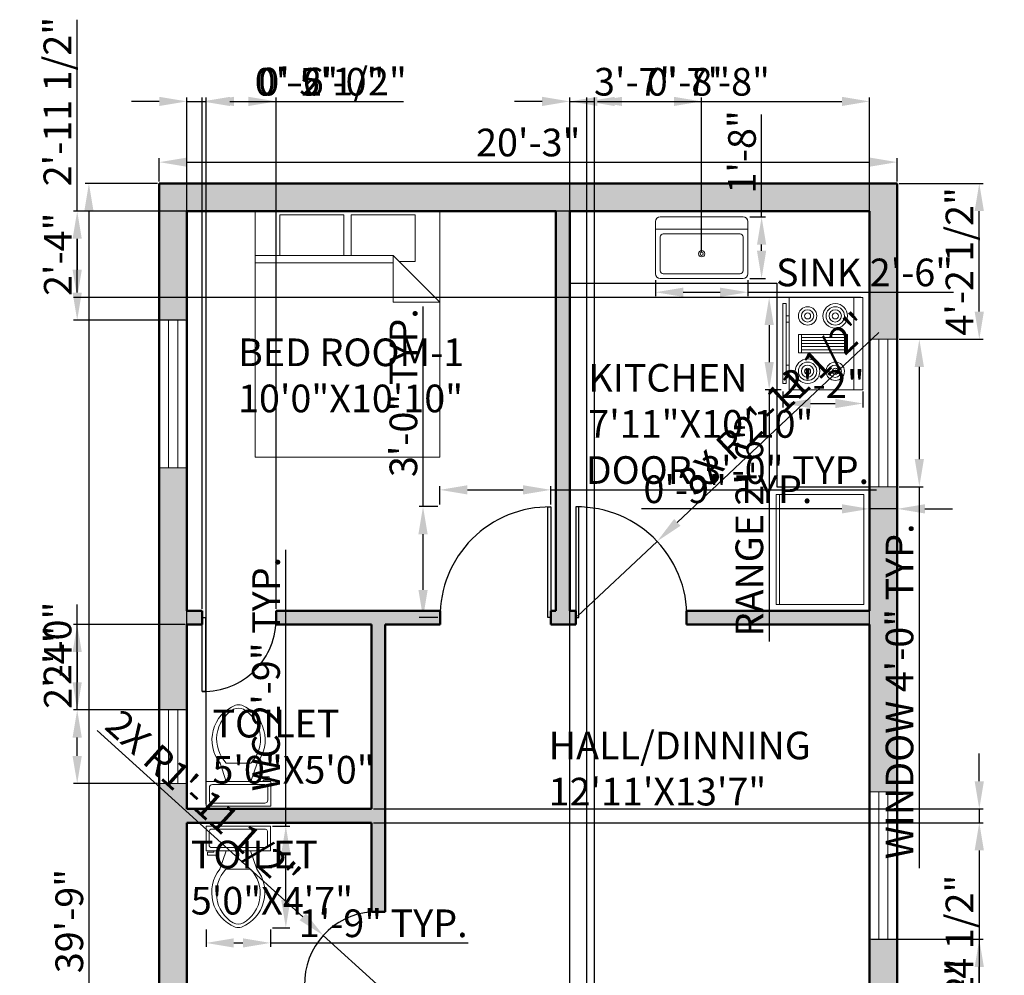
# Model space of a CAD drawing. Units: inches. Extents: x 66818 to 67138, y 29633 to 30215.
# Tile 2 of 2: x 66818 to 67138, y 29904 to 30215. Entities that reach past the tile are written whole.
import ezdxf

# ---------------------------------------------------------------- set-up
doc = ezdxf.new("R2010")
doc.units = ezdxf.units.IN
for name, color, linetype, lineweight in [('A-ANNO-DIMS', 2, 'Continuous', 18), ('A-AREA-IDEN', 7, 'Continuous', 25), ('A-DOOR', 3, 'Continuous', 25), ('A-EQPM', 8, 'Continuous', 18), ('A-FLOR-CASE', 8, 'Continuous', 25), ('A-FLOR-FIXT', 9, 'Continuous', 18), ('A-FURN', 8, 'Continuous', 18), ('A-GLAZ', 4, 'Continuous', 18), ('A-WALL', 7, 'Continuous', 50)]:
    doc.layers.add(name, color=color, linetype=linetype, lineweight=lineweight)
doc.layers.add('A-WALL-PATT', color=251, linetype='Continuous', lineweight=13, true_color=0x636466)
doc.styles.get("Standard").update_dxf_attribs({"font": 'arial.ttf'})
doc.dimstyles.new('ISO-25', dxfattribs={"dimtxt": 9, "dimasz": 9, "dimexe": 1.25, "dimexo": 0.625, "dimtad": 1, "dimdec": 1, "dimrnd": 9, "dimlunit": 3, "dimtxsty": 'Standard', "dimcen": 2.5, "dimadec": 0, "dimazin": 0, "dimtfac": 1, "dimtdec": 1, "dimtmove": 0, "dimatfit": 3, "dimfxl": 1, "dimarcsym": 0})

# ---------------------------------------------------------------- blocks, each defined once
blk = doc.blocks.new('Bed - Queen')
for p, q in [((0, -80.00003), (0, 0)), ((0, 0), (59.99999, 0)), ((59.99999, 0), (59.99999, -80.00003)), ((7.99999, -1.2), (28.79998, -1.2)), ((7.99999, -14.4), (7.99999, -1.2)), ((28.79998, -1.2), (28.79998, -14.4)), ((31.19999, -1.2), (51.99999, -1.2)), ((31.19999, -14.4), (31.19999, -1.2)), ((51.99999, -1.2), (51.99999, -16.4)), ((0, -14.4), (44.8, -14.4)), ((59.99999, -29.6), (44.8, -14.4)), ((44.8, -14.4), (44.8, -29.6)), ((44.8, -16.8), (0, -16.8)), ((51.99999, -16.4), (46.79936, -16.4)), ((44.8, -29.6), (59.99999, -29.6)), ((59.99999, -80.00003), (0, -80.00003))]:
    blk.add_line(p, q)
blk = doc.blocks.new('Toilet - top')
for p, q in [((9.5, -6), (9.5, -2)), ((-10, -8.5), (-8, -8.5)), ((-10, -9.5), (-10, -8.5)), ((-7, -9.5), (-10, -9.5)), ((-8, -8.5), (-8, -8)), ((-7, -8), (-7, -9.5)), ((-4, -8), (-6, -14)), ((4, -8), (6, -14)), ((4, -14), (-4, -14))]:
    blk.add_line(p, q)
blk.add_lwpolyline([(10.5, -8), (10.5, 0), (-10.5, 0), (-10.5, -8)], close=True)
for points in [[(-9.5, -2), (-9.5, -6)], [(8.5, -1), (-8.5, -1)], [(-8.5, -7), (8.5, -7)]]:
    blk.add_lwpolyline(points)
for centre, radius, start, end in [((-8.62, -1.88), 0.884, 81.8699, 188.1301), ((8.62, -1.88), 0.884, 351.8699, 98.1301), ((-8.62, -6.12), 0.884, 171.8699, 278.1301), ((8.62, -6.12), 0.884, 261.8699, 8.1301), ((3.52, -21.58), 12.17, 141.4691, 247.9714), ((4.2, -21.82), 11.33, 136.3677, 238.9468), ((-3.52, -21.58), 12.17, 292.0284, 38.5307), ((-4.2, -21.82), 11.33, 301.053, 43.6321), ((0, -27.88), 4, 245.7318, 294.2682), ((0, -29), 4, 254.8605, 285.1395)]:
    blk.add_arc(centre, radius, start, end)
blk = doc.blocks.new('Sink-single - 30 in top')
blk.add_line((-15, -3.999996), (15, -3.999996))
for points in [[(-13.5, 0), (13.5, 0)], [(-15, -18.499996), (-15, -1.5)], [(15, -1.5), (15, -18.499996)], [(-12.5, -5.499996), (12.5, -5.499996)], [(-13.5, -17.499996), (-13.5, -6.499996)], [(13.5, -6.499996), (13.5, -17.499996)], [(12.5, -18.499996), (-12.5, -18.499996)], [(13.5, -19.999996), (-13.5, -19.999996)]]:
    blk.add_lwpolyline(points)
for radius in [1, 0.5]:
    blk.add_circle((0, -11.999996), radius)
for centre, radius, start, end in [((-13.5, -1.5), 1.5, 90, 180), ((13.5, -1.5), 1.5, 0, 90), ((-12.5, -6.499996), 1, 90, 180), ((12.5, -6.499996), 1, 0, 90), ((-13.5, -18.499996), 1.5, 180, 270), ((-12.5, -17.499996), 1, 180, 270), ((12.5, -17.499996), 1, 270, 0), ((13.5, -18.499996), 1.5, 270, 0)]:
    blk.add_arc(centre, radius, start, end)
blk = doc.blocks.new('*D9')
at = {"layer": 'A-ANNO-DIMS', "color": 0, "lineweight": -2, "transparency": 16777216}
for p, q in [((66863.23, 30162.54), (66863.23, 30170.1)), ((67103.23, 30162.54), (67103.23, 30170.1)), ((66872.23, 30168.85), (67094.23, 30168.85))]:
    blk.add_line(p, q, dxfattribs=at)
at = {"layer": 'A-ANNO-DIMS', "color": 0, "transparency": 16777216}
for points in [[(66872.23, 30170.35), (66872.23, 30167.35), (66863.23, 30168.85)], [(67094.23, 30170.35), (67094.23, 30167.35), (67103.23, 30168.85)]]:
    blk.add_solid(points, dxfattribs=at)
at = {"layer": 'Defpoints', "color": 0, "transparency": 16777216}
for p in [(67103.23, 30168.85), (66863.23, 30161.91), (67103.23, 30161.91)]:
    blk.add_point(p, dxfattribs=at)
at = {"layer": 'A-ANNO-DIMS', "color": 0, "transparency": 16777216, "insert": (66983.23, 30174.07), "char_height": 9, "attachment_point": 5}
blk.add_mtext('20\'-3"', dxfattribs=at)
blk = doc.blocks.new('*D10')
at = {"layer": 'A-ANNO-DIMS', "color": 0, "lineweight": -2, "transparency": 16777216}
for p, q in [((66862.6, 30161.91), (66839.1, 30161.91)), ((66840.35, 30152.91), (66840.35, 29690.91)), ((66862.6, 29681.91), (66839.1, 29681.91))]:
    blk.add_line(p, q, dxfattribs=at)
at = {"layer": 'A-ANNO-DIMS', "color": 0, "transparency": 16777216}
for points in [[(66838.85, 30152.91), (66841.85, 30152.91), (66840.35, 30161.91)], [(66838.85, 29690.91), (66841.85, 29690.91), (66840.35, 29681.91)]]:
    blk.add_solid(points, dxfattribs=at)
at = {"layer": 'Defpoints', "color": 0, "transparency": 16777216}
for p in [(66863.23, 30161.91), (66840.35, 29681.91), (66863.23, 29681.91)]:
    blk.add_point(p, dxfattribs=at)
at = {"layer": 'A-ANNO-DIMS', "color": 0, "transparency": 16777216, "insert": (66835.13, 29921.91), "char_height": 9, "attachment_point": 5, "rotation": 90}
blk.add_mtext('39\'-9"', dxfattribs=at)
blk = doc.blocks.new('Range-Oven - 30 in top')
for p, q in [((0, -3), (30, -3)), ((12, -6), (18, -6)), ((13, -20), (13, -6)), ((14, -6), (14, -20)), ((15, -20), (15, -6)), ((16, -6), (16, -20)), ((17, -20), (17, -6)), ((18, -20), (12, -20)), ((6, -24), (6, -25)), ((8, -25), (8, -24)), ((22, -25), (22, -24)), ((24, -24), (24, -25))]:
    blk.add_line(p, q)
for points in [[(0, -24), (0, 0), (30, 0), (30, -24)], [(12, -21), (12, -5), (18, -5), (18, -21)], [(2, -26), (2, -25), (28, -25), (28, -26)]]:
    blk.add_lwpolyline(points, close=True)
for centre, radius in [((6, -9), 4), ((6, -9), 3), ((24, -9), 3), ((6, -9), 2), ((6, -9), 1), ((24, -9), 2), ((24, -9), 1), ((6, -18), 3), ((6, -18), 2), ((24, -18), 4), ((24, -18), 3), ((24, -18), 2), ((6, -18), 1), ((24, -18), 1)]:
    blk.add_circle(centre, radius)
blk = doc.blocks.new('WIN-48IN')
for p, q in [((9, 48), (0, 48)), ((3, 48), (3, 0)), ((6, 48), (6, 0)), ((9, 0), (0, 0))]:
    blk.add_line(p, q)
blk = doc.blocks.new('DOOR-SWING-36IN')
for p, q in [((35, 0), (35, 36)), ((35, 36), (36, 36)), ((36, 36), (36, 2.25)), ((36, 0), (35, 0))]:
    blk.add_line(p, q)
blk.add_arc((35.5, 0.5), 35.5, 89.1931, 180.8069)
blk = doc.blocks.new('*D13')
at = {"layer": 'A-ANNO-DIMS', "color": 0, "lineweight": -2, "transparency": 16777216}
for p, q in [((67103.85, 30111.23), (67111.68, 30111.23)), ((67110.43, 30102.23), (67110.43, 30072.23)), ((67103.85, 30063.23), (67111.68, 30063.23)), ((67110.43, 30063.23), (67110.43, 29939.1))]:
    blk.add_line(p, q, dxfattribs=at)
at = {"layer": 'A-ANNO-DIMS', "color": 0, "transparency": 16777216}
for points in [[(67108.93, 30102.23), (67111.93, 30102.23), (67110.43, 30111.23)], [(67108.93, 30072.23), (67111.93, 30072.23), (67110.43, 30063.23)]]:
    blk.add_solid(points, dxfattribs=at)
at = {"layer": 'Defpoints', "color": 0, "transparency": 16777216}
for p in [(67103.23, 30111.23), (67103.23, 30063.23), (67110.43, 30063.23)]:
    blk.add_point(p, dxfattribs=at)
at = {"layer": 'A-ANNO-DIMS', "color": 0, "transparency": 16777216, "insert": (67105.15, 29996.66), "char_height": 9, "attachment_point": 5, "rotation": 90}
blk.add_mtext('WINDOW 4\'-0" TYP.', dxfattribs=at)
blk = doc.blocks.new('*D14')
at = {"layer": 'A-ANNO-DIMS', "color": 0, "lineweight": -2, "transparency": 16777216}
for p, q in [((67094.23, 30062.61), (67094.23, 30054.78)), ((67103.23, 30062.61), (67103.23, 30054.78)), ((67085.23, 30056.03), (67020.12, 30056.03)), ((67103.23, 30056.03), (67094.23, 30056.03)), ((67112.23, 30056.03), (67121.23, 30056.03))]:
    blk.add_line(p, q, dxfattribs=at)
at = {"layer": 'A-ANNO-DIMS', "color": 0, "transparency": 16777216}
for points in [[(67085.23, 30057.53), (67085.23, 30054.53), (67094.23, 30056.03)], [(67112.23, 30057.53), (67112.23, 30054.53), (67103.23, 30056.03)]]:
    blk.add_solid(points, dxfattribs=at)
at = {"layer": 'Defpoints', "color": 0, "transparency": 16777216}
for p in [(67094.23, 30063.23), (67103.23, 30063.23), (67094.23, 30056.03)]:
    blk.add_point(p, dxfattribs=at)
at = {"layer": 'A-ANNO-DIMS', "color": 0, "transparency": 16777216, "insert": (67048.17, 30061.25), "char_height": 9, "attachment_point": 5}
blk.add_mtext('0\'-9" TYP.', dxfattribs=at)
blk = doc.blocks.new('*D17')
at = {"layer": 'A-ANNO-DIMS', "color": 0, "lineweight": -2, "transparency": 16777216}
for p, q in [((66904.39, 29952.81), (66904.39, 30042.72)), ((66900.06, 29952.81), (66905.64, 29952.81)), ((66904.39, 29928.76), (66904.39, 29943.81)), ((66900.06, 29919.76), (66905.64, 29919.76))]:
    blk.add_line(p, q, dxfattribs=at)
at = {"layer": 'A-ANNO-DIMS', "color": 0, "transparency": 16777216}
for points in [[(66902.89, 29943.81), (66905.89, 29943.81), (66904.39, 29952.81)], [(66902.89, 29928.76), (66905.89, 29928.76), (66904.39, 29919.76)]]:
    blk.add_solid(points, dxfattribs=at)
at = {"layer": 'Defpoints', "color": 0, "transparency": 16777216}
for p in [(66899.43, 29952.81), (66904.39, 29952.81), (66899.43, 29919.76)]:
    blk.add_point(p, dxfattribs=at)
at = {"layer": 'A-ANNO-DIMS', "color": 0, "transparency": 16777216, "insert": (66899.11, 30002.26), "char_height": 9, "attachment_point": 5, "rotation": 90}
blk.add_mtext('WC 2\'-9" TYP.', dxfattribs=at)
blk = doc.blocks.new('*D18')
at = {"layer": 'A-ANNO-DIMS', "color": 0, "lineweight": -2, "transparency": 16777216}
for p, q in [((66878.43, 29919.13), (66878.43, 29913.55)), ((66899.43, 29919.13), (66899.43, 29913.55)), ((66887.43, 29914.8), (66890.43, 29914.8)), ((66899.43, 29914.8), (66963.7, 29914.8))]:
    blk.add_line(p, q, dxfattribs=at)
at = {"layer": 'A-ANNO-DIMS', "color": 0, "transparency": 16777216}
for points in [[(66887.43, 29916.3), (66887.43, 29913.3), (66878.43, 29914.8)], [(66890.43, 29916.3), (66890.43, 29913.3), (66899.43, 29914.8)]]:
    blk.add_solid(points, dxfattribs=at)
at = {"layer": 'Defpoints', "color": 0, "transparency": 16777216}
for p in [(66878.43, 29919.76), (66899.43, 29919.76), (66899.43, 29914.8)]:
    blk.add_point(p, dxfattribs=at)
at = {"layer": 'A-ANNO-DIMS', "color": 0, "transparency": 16777216, "insert": (66936.06, 29920.02), "char_height": 9, "attachment_point": 5}
blk.add_mtext('1\'-9" TYP.', dxfattribs=at)
blk = doc.blocks.new('*D19')
at = {"layer": 'A-ANNO-DIMS', "color": 0, "lineweight": -2, "transparency": 16777216}
for p, q in [((66954.44, 30057.42), (66954.44, 30063.47)), ((66963.44, 30062.22), (66981.58, 30062.22)), ((66990.58, 30057.42), (66990.58, 30063.47)), ((66990.58, 30062.22), (67096.45, 30062.22))]:
    blk.add_line(p, q, dxfattribs=at)
at = {"layer": 'A-ANNO-DIMS', "color": 0, "transparency": 16777216}
for points in [[(66963.44, 30063.72), (66963.44, 30060.72), (66954.44, 30062.22)], [(66981.58, 30063.72), (66981.58, 30060.72), (66990.58, 30062.22)]]:
    blk.add_solid(points, dxfattribs=at)
at = {"layer": 'Defpoints', "color": 0, "transparency": 16777216}
for p in [(66990.58, 30062.22), (66954.44, 30056.8), (66990.58, 30056.8)]:
    blk.add_point(p, dxfattribs=at)
at = {"layer": 'A-ANNO-DIMS', "color": 0, "transparency": 16777216, "insert": (67048.01, 30067.5), "char_height": 9, "attachment_point": 5}
blk.add_mtext('DOOR 3\'-0" TYP.', dxfattribs=at)
blk = doc.blocks.new('*D20')
at = {"layer": 'A-ANNO-DIMS', "color": 0, "lineweight": -2, "transparency": 16777216}
for p, q in [((66949.02, 30056.8), (66949.02, 30121.9)), ((66953.82, 30056.8), (66947.77, 30056.8)), ((66949.02, 30029.66), (66949.02, 30047.8)), ((66953.82, 30020.66), (66947.77, 30020.66))]:
    blk.add_line(p, q, dxfattribs=at)
at = {"layer": 'A-ANNO-DIMS', "color": 0, "transparency": 16777216}
for points in [[(66947.52, 30047.8), (66950.52, 30047.8), (66949.02, 30056.8)], [(66947.52, 30029.66), (66950.52, 30029.66), (66949.02, 30020.66)]]:
    blk.add_solid(points, dxfattribs=at)
at = {"layer": 'Defpoints', "color": 0, "transparency": 16777216}
for p in [(66949.02, 30056.8), (66954.44, 30056.8), (66954.44, 30020.66)]:
    blk.add_point(p, dxfattribs=at)
at = {"layer": 'A-ANNO-DIMS', "color": 0, "transparency": 16777216, "insert": (66943.8, 30093.85), "char_height": 9, "attachment_point": 5, "rotation": 90}
blk.add_mtext('3\'-0" TYP.', dxfattribs=at)
blk = doc.blocks.new('*D21')
at = {"layer": 'A-ANNO-DIMS', "color": 0, "lineweight": -2, "transparency": 16777216}
for p, q in [((67024.63, 30130.4), (67024.63, 30125.27)), ((67054.63, 30130.4), (67054.63, 30125.27)), ((67033.63, 30126.52), (67045.63, 30126.52)), ((67054.63, 30126.52), (67121.6, 30126.52))]:
    blk.add_line(p, q, dxfattribs=at)
at = {"layer": 'A-ANNO-DIMS', "color": 0, "transparency": 16777216}
for points in [[(67033.63, 30128.02), (67033.63, 30125.02), (67024.63, 30126.52)], [(67045.63, 30128.02), (67045.63, 30125.02), (67054.63, 30126.52)]]:
    blk.add_solid(points, dxfattribs=at)
at = {"layer": 'Defpoints', "color": 0, "transparency": 16777216}
for p in [(67024.63, 30131.02), (67054.63, 30131.02), (67054.63, 30126.52)]:
    blk.add_point(p, dxfattribs=at)
at = {"layer": 'A-ANNO-DIMS', "color": 0, "transparency": 16777216, "insert": (67092.62, 30131.8), "char_height": 9, "attachment_point": 5}
blk.add_mtext('SINK 2\'-6"', dxfattribs=at)
blk = doc.blocks.new('*D22')
at = {"layer": 'A-ANNO-DIMS', "color": 0, "lineweight": -2, "transparency": 16777216}
for p, q in [((67059.13, 30151.02), (67059.13, 30184.35)), ((67055.26, 30151.02), (67060.38, 30151.02)), ((67059.13, 30140.02), (67059.13, 30142.02)), ((67055.26, 30131.02), (67060.38, 30131.02))]:
    blk.add_line(p, q, dxfattribs=at)
at = {"layer": 'A-ANNO-DIMS', "color": 0, "transparency": 16777216}
for points in [[(67057.63, 30142.02), (67060.63, 30142.02), (67059.13, 30151.02)], [(67057.63, 30140.02), (67060.63, 30140.02), (67059.13, 30131.02)]]:
    blk.add_solid(points, dxfattribs=at)
at = {"layer": 'Defpoints', "color": 0, "transparency": 16777216}
for p in [(67054.63, 30151.02), (67059.13, 30151.02), (67054.63, 30131.02)]:
    blk.add_point(p, dxfattribs=at)
at = {"layer": 'A-ANNO-DIMS', "color": 0, "transparency": 16777216, "insert": (67053.91, 30172.19), "char_height": 9, "attachment_point": 5, "rotation": 90}
blk.add_mtext('1\'-8"', dxfattribs=at)
blk = doc.blocks.new('*D23')
at = {"layer": 'A-ANNO-DIMS', "color": 0, "lineweight": -2, "transparency": 16777216}
for p, q in [((67065.46, 30124.82), (67060.34, 30124.82)), ((67061.59, 30115.82), (67061.59, 30103.82)), ((67065.46, 30094.82), (67060.34, 30094.82)), ((67061.59, 30094.82), (67061.59, 30012.9))]:
    blk.add_line(p, q, dxfattribs=at)
at = {"layer": 'A-ANNO-DIMS', "color": 0, "transparency": 16777216}
for points in [[(67060.09, 30115.82), (67063.09, 30115.82), (67061.59, 30124.82)], [(67060.09, 30103.82), (67063.09, 30103.82), (67061.59, 30094.82)]]:
    blk.add_solid(points, dxfattribs=at)
at = {"layer": 'Defpoints', "color": 0, "transparency": 16777216}
for p in [(67066.09, 30124.82), (67061.59, 30094.82), (67066.09, 30094.82)]:
    blk.add_point(p, dxfattribs=at)
at = {"layer": 'A-ANNO-DIMS', "color": 0, "transparency": 16777216, "insert": (67056.31, 30049.36), "char_height": 9, "attachment_point": 5, "rotation": 90}
blk.add_mtext('RANGE 2\'-6"', dxfattribs=at)
blk = doc.blocks.new('*D24')
at = {"layer": 'A-ANNO-DIMS', "color": 0, "lineweight": -2, "transparency": 16777216}
for p, q in [((67066.09, 30094.19), (67066.09, 30089.07)), ((67092.09, 30094.19), (67092.09, 30089.07)), ((67075.09, 30090.32), (67083.09, 30090.32))]:
    blk.add_line(p, q, dxfattribs=at)
at = {"layer": 'A-ANNO-DIMS', "color": 0, "transparency": 16777216}
for points in [[(67075.09, 30091.82), (67075.09, 30088.82), (67066.09, 30090.32)], [(67083.09, 30091.82), (67083.09, 30088.82), (67092.09, 30090.32)]]:
    blk.add_solid(points, dxfattribs=at)
at = {"layer": 'Defpoints', "color": 0, "transparency": 16777216}
for p in [(67066.09, 30094.82), (67092.09, 30094.82), (67092.09, 30090.32)]:
    blk.add_point(p, dxfattribs=at)
at = {"layer": 'A-ANNO-DIMS', "color": 0, "transparency": 16777216, "insert": (67079.09, 30095.46), "char_height": 9, "attachment_point": 5}
blk.add_mtext('2\'-2"', dxfattribs=at)
blk = doc.blocks.new('*D27')
at = {"layer": 'A-ANNO-DIMS', "color": 0, "lineweight": -2, "transparency": 16777216}
for p, q in [((66877.23, 30023.54), (66877.23, 30189.86)), ((66901.23, 30023.54), (66901.23, 30189.86)), ((66886.23, 30188.61), (66892.23, 30188.61)), ((66901.23, 30188.61), (66935.55, 30188.61))]:
    blk.add_line(p, q, dxfattribs=at)
at = {"layer": 'A-ANNO-DIMS', "color": 0, "transparency": 16777216}
for points in [[(66886.23, 30190.11), (66886.23, 30187.11), (66877.23, 30188.61)], [(66892.23, 30190.11), (66892.23, 30187.11), (66901.23, 30188.61)]]:
    blk.add_solid(points, dxfattribs=at)
at = {"layer": 'Defpoints', "color": 0, "transparency": 16777216}
for p in [(66901.23, 30188.61), (66877.23, 30022.91), (66901.23, 30022.91)]:
    blk.add_point(p, dxfattribs=at)
at = {"layer": 'A-ANNO-DIMS', "color": 0, "transparency": 16777216, "insert": (66922.89, 30193.83), "char_height": 9, "attachment_point": 5}
blk.add_mtext('2\'-0"', dxfattribs=at)
blk = doc.blocks.new('*D28')
at = {"layer": 'A-ANNO-DIMS', "color": 0, "lineweight": -2, "transparency": 16777216}
for p, q in [((66872.23, 30023.54), (66872.23, 30189.86)), ((66877.23, 30023.54), (66877.23, 30189.86)), ((66863.23, 30188.61), (66854.23, 30188.61)), ((66872.23, 30188.61), (66877.23, 30188.61)), ((66886.23, 30188.61), (66920.4, 30188.61))]:
    blk.add_line(p, q, dxfattribs=at)
at = {"layer": 'A-ANNO-DIMS', "color": 0, "transparency": 16777216}
for points in [[(66863.23, 30190.11), (66863.23, 30187.11), (66872.23, 30188.61)], [(66886.23, 30190.11), (66886.23, 30187.11), (66877.23, 30188.61)]]:
    blk.add_solid(points, dxfattribs=at)
at = {"layer": 'Defpoints', "color": 0, "transparency": 16777216}
for p in [(66877.23, 30188.61), (66872.23, 30022.91), (66877.23, 30022.91)]:
    blk.add_point(p, dxfattribs=at)
at = {"layer": 'A-ANNO-DIMS', "color": 0, "transparency": 16777216, "insert": (66907.81, 30193.83), "char_height": 9, "attachment_point": 5}
blk.add_mtext('0\'-5"', dxfattribs=at)
blk = doc.blocks.new('*D29')
at = {"layer": 'A-ANNO-DIMS', "color": 0, "lineweight": -2, "transparency": 16777216}
for p, q in [((67129.93, 29967.41), (67129.93, 29976.41)), ((66932.85, 29958.41), (67131.18, 29958.41)), ((67129.93, 29958.41), (67129.93, 29953.91)), ((66932.85, 29953.91), (67131.18, 29953.91)), ((67129.93, 29944.91), (67129.93, 29889.77))]:
    blk.add_line(p, q, dxfattribs=at)
at = {"layer": 'A-ANNO-DIMS', "color": 0, "transparency": 16777216}
for points in [[(67128.43, 29967.41), (67131.43, 29967.41), (67129.93, 29958.41)], [(67128.43, 29944.91), (67131.43, 29944.91), (67129.93, 29953.91)]]:
    blk.add_solid(points, dxfattribs=at)
at = {"layer": 'Defpoints', "color": 0, "transparency": 16777216}
for p in [(66932.23, 29958.41), (66932.23, 29953.91), (67129.93, 29953.91)]:
    blk.add_point(p, dxfattribs=at)
at = {"layer": 'A-ANNO-DIMS', "color": 0, "transparency": 16777216, "insert": (67124.65, 29912.84), "char_height": 9, "attachment_point": 5, "rotation": 90}
blk.add_mtext('0\'-4 1/2"', dxfattribs=at)
blk = doc.blocks.new('*D30')
at = {"layer": 'A-ANNO-DIMS', "color": 0, "lineweight": -2, "transparency": 16777216}
for p, q in [((66836.53, 30152.91), (66836.53, 30215.21)), ((66871.6, 30152.91), (66835.28, 30152.91)), ((66836.53, 30126.42), (66836.53, 30143.91)), ((66871.6, 30117.42), (66835.28, 30117.42))]:
    blk.add_line(p, q, dxfattribs=at)
at = {"layer": 'A-ANNO-DIMS', "color": 0, "transparency": 16777216}
for points in [[(66835.03, 30143.91), (66838.03, 30143.91), (66836.53, 30152.91)], [(66835.03, 30126.42), (66838.03, 30126.42), (66836.53, 30117.42)]]:
    blk.add_solid(points, dxfattribs=at)
at = {"layer": 'Defpoints', "color": 0, "transparency": 16777216}
for p in [(66836.53, 30152.91), (66872.23, 30152.91), (66872.23, 30117.42)]:
    blk.add_point(p, dxfattribs=at)
at = {"layer": 'A-ANNO-DIMS', "color": 0, "transparency": 16777216, "insert": (66831.25, 30188.56), "char_height": 9, "attachment_point": 5, "rotation": 90}
blk.add_mtext('2\'-11 1/2"', dxfattribs=at)
blk = doc.blocks.new('*D31')
at = {"layer": 'A-ANNO-DIMS', "color": 0, "lineweight": -2, "transparency": 16777216}
for p, q in [((67103.85, 30161.91), (67131.18, 30161.91)), ((67129.93, 30120.23), (67129.93, 30152.91)), ((67103.85, 30111.23), (67131.18, 30111.23))]:
    blk.add_line(p, q, dxfattribs=at)
at = {"layer": 'A-ANNO-DIMS', "color": 0, "transparency": 16777216}
for points in [[(67128.43, 30152.91), (67131.43, 30152.91), (67129.93, 30161.91)], [(67128.43, 30120.23), (67131.43, 30120.23), (67129.93, 30111.23)]]:
    blk.add_solid(points, dxfattribs=at)
at = {"layer": 'Defpoints', "color": 0, "transparency": 16777216}
for p in [(67103.23, 30161.91), (67129.93, 30161.91), (67103.23, 30111.23)]:
    blk.add_point(p, dxfattribs=at)
at = {"layer": 'A-ANNO-DIMS', "color": 0, "transparency": 16777216, "insert": (67124.65, 30136.57), "char_height": 9, "attachment_point": 5, "rotation": 90}
blk.add_mtext('4\'-2 1/2"', dxfattribs=at)
blk = doc.blocks.new('*D32')
at = {"layer": 'A-ANNO-DIMS', "color": 0, "lineweight": -2, "transparency": 16777216}
for p, q in [((67094.85, 29915.99), (67131.18, 29915.99)), ((67129.93, 29864.41), (67129.93, 29906.99)), ((67094.85, 29855.41), (67131.18, 29855.41))]:
    blk.add_line(p, q, dxfattribs=at)
at = {"layer": 'A-ANNO-DIMS', "color": 0, "transparency": 16777216}
for points in [[(67128.43, 29906.99), (67131.43, 29906.99), (67129.93, 29915.99)], [(67128.43, 29864.41), (67131.43, 29864.41), (67129.93, 29855.41)]]:
    blk.add_solid(points, dxfattribs=at)
at = {"layer": 'Defpoints', "color": 0, "transparency": 16777216}
for p in [(67094.23, 29915.99), (67129.93, 29915.99), (67094.23, 29855.41)]:
    blk.add_point(p, dxfattribs=at)
at = {"layer": 'A-ANNO-DIMS', "color": 0, "transparency": 16777216, "insert": (67124.65, 29885.7), "char_height": 9, "attachment_point": 5, "rotation": 90}
blk.add_mtext('5\'-0 1/2"', dxfattribs=at)
blk = doc.blocks.new('*D33')
at = {"layer": 'A-ANNO-DIMS', "color": 0, "lineweight": -2, "transparency": 16777216}
for p, q in [((66871.6, 30018.41), (66835.28, 30018.41)), ((66836.53, 30009.41), (66836.53, 29999.63)), ((66871.6, 29990.63), (66835.28, 29990.63))]:
    blk.add_line(p, q, dxfattribs=at)
at = {"layer": 'A-ANNO-DIMS', "color": 0, "transparency": 16777216}
for points in [[(66835.03, 30009.41), (66838.03, 30009.41), (66836.53, 30018.41)], [(66835.03, 29999.63), (66838.03, 29999.63), (66836.53, 29990.63)]]:
    blk.add_solid(points, dxfattribs=at)
at = {"layer": 'Defpoints', "color": 0, "transparency": 16777216}
for p in [(66872.23, 30018.41), (66836.53, 29990.63), (66872.23, 29990.63)]:
    blk.add_point(p, dxfattribs=at)
at = {"layer": 'A-ANNO-DIMS', "color": 0, "transparency": 16777216, "insert": (66831.39, 30004.52), "char_height": 9, "attachment_point": 5, "rotation": 90}
blk.add_mtext('2\'-4"', dxfattribs=at)
blk = doc.blocks.new('*D34')
at = {"layer": 'A-ANNO-DIMS', "color": 0, "lineweight": -2, "transparency": 16777216}
for p, q in [((66836.53, 29990.63), (66836.53, 30024.96)), ((66862.6, 29990.63), (66835.28, 29990.63)), ((66836.53, 29975.63), (66836.53, 29981.63)), ((66862.6, 29966.63), (66835.28, 29966.63))]:
    blk.add_line(p, q, dxfattribs=at)
at = {"layer": 'A-ANNO-DIMS', "color": 0, "transparency": 16777216}
for points in [[(66835.03, 29981.63), (66838.03, 29981.63), (66836.53, 29990.63)], [(66835.03, 29975.63), (66838.03, 29975.63), (66836.53, 29966.63)]]:
    blk.add_solid(points, dxfattribs=at)
at = {"layer": 'Defpoints', "color": 0, "transparency": 16777216}
for p in [(66836.53, 29990.63), (66863.23, 29990.63), (66863.23, 29966.63)]:
    blk.add_point(p, dxfattribs=at)
at = {"layer": 'A-ANNO-DIMS', "color": 0, "transparency": 16777216, "insert": (66831.31, 30012.29), "char_height": 9, "attachment_point": 5, "rotation": 90}
blk.add_mtext('2\'-0"', dxfattribs=at)
blk = doc.blocks.new('*D40')
at = {"layer": 'A-ANNO-DIMS', "color": 0, "lineweight": -2, "transparency": 16777216}
for p, q in [((66996.73, 30153.54), (66996.73, 30189.86)), ((67039.63, 30139.65), (67039.63, 30189.86)), ((67005.73, 30188.61), (67030.63, 30188.61))]:
    blk.add_line(p, q, dxfattribs=at)
at = {"layer": 'A-ANNO-DIMS', "color": 0, "transparency": 16777216}
for points in [[(67005.73, 30190.11), (67005.73, 30187.11), (66996.73, 30188.61)], [(67030.63, 30190.11), (67030.63, 30187.11), (67039.63, 30188.61)]]:
    blk.add_solid(points, dxfattribs=at)
at = {"layer": 'Defpoints', "color": 0, "transparency": 16777216}
for p in [(67039.63, 30188.61), (66996.73, 30152.91), (67039.63, 30139.02)]:
    blk.add_point(p, dxfattribs=at)
at = {"layer": 'A-ANNO-DIMS', "color": 0, "transparency": 16777216, "insert": (67018.18, 30193.84), "char_height": 9, "attachment_point": 5}
blk.add_mtext('3\'-7"', dxfattribs=at)
blk = doc.blocks.new('*D41')
at = {"layer": 'A-ANNO-DIMS', "color": 0, "lineweight": -2, "transparency": 16777216}
for p, q in [((67093.6, 30152.91), (66835.28, 30152.91)), ((66836.53, 30143.91), (66836.53, 30133.82)), ((67091.46, 30124.82), (66835.28, 30124.82))]:
    blk.add_line(p, q, dxfattribs=at)
at = {"layer": 'A-ANNO-DIMS', "color": 0, "transparency": 16777216}
for points in [[(66835.03, 30143.91), (66838.03, 30143.91), (66836.53, 30152.91)], [(66835.03, 30133.82), (66838.03, 30133.82), (66836.53, 30124.82)]]:
    blk.add_solid(points, dxfattribs=at)
at = {"layer": 'Defpoints', "color": 0, "transparency": 16777216}
for p in [(67094.23, 30152.91), (66836.53, 30124.82), (67092.09, 30124.82)]:
    blk.add_point(p, dxfattribs=at)
at = {"layer": 'A-ANNO-DIMS', "color": 0, "transparency": 16777216, "insert": (66831.39, 30138.87), "char_height": 9, "attachment_point": 5, "rotation": 90}
blk.add_mtext('2\'-4"', dxfattribs=at)
blk = doc.blocks.new('*D42')
at = {"layer": 'A-ANNO-DIMS', "color": 0, "lineweight": -2, "transparency": 16777216}
for p, q in [((66872.23, 29959.04), (66872.23, 30189.86)), ((66878.52, 29959.92), (66878.52, 30189.86)), ((66863.23, 30188.61), (66854.23, 30188.61)), ((66872.23, 30188.61), (66878.52, 30188.61)), ((66887.52, 30188.61), (66942.67, 30188.61))]:
    blk.add_line(p, q, dxfattribs=at)
at = {"layer": 'A-ANNO-DIMS', "color": 0, "transparency": 16777216}
for points in [[(66863.23, 30190.11), (66863.23, 30187.11), (66872.23, 30188.61)], [(66887.52, 30190.11), (66887.52, 30187.11), (66878.52, 30188.61)]]:
    blk.add_solid(points, dxfattribs=at)
at = {"layer": 'Defpoints', "color": 0, "transparency": 16777216}
for p in [(66878.52, 30188.61), (66878.52, 29959.3), (66872.23, 29958.41)]:
    blk.add_point(p, dxfattribs=at)
at = {"layer": 'A-ANNO-DIMS', "color": 0, "transparency": 16777216, "insert": (66919.59, 30193.89), "char_height": 9, "attachment_point": 5}
blk.add_mtext('0\'-6 1/2"', dxfattribs=at)
blk = doc.blocks.new('*D43')
at = {"layer": 'A-ANNO-DIMS', "color": 0, "lineweight": -2, "transparency": 16777216}
for p, q in [((67002.34, 29682.54), (67002.34, 30189.86)), ((67094.23, 29682.54), (67094.23, 30189.86)), ((67011.34, 30188.61), (67085.23, 30188.61))]:
    blk.add_line(p, q, dxfattribs=at)
at = {"layer": 'A-ANNO-DIMS', "color": 0, "transparency": 16777216}
for points in [[(67011.34, 30190.11), (67011.34, 30187.11), (67002.34, 30188.61)], [(67085.23, 30190.11), (67085.23, 30187.11), (67094.23, 30188.61)]]:
    blk.add_solid(points, dxfattribs=at)
at = {"layer": 'Defpoints', "color": 0, "transparency": 16777216}
for p in [(67094.23, 30188.61), (67002.34, 29681.91), (67094.23, 29681.91)]:
    blk.add_point(p, dxfattribs=at)
at = {"layer": 'A-ANNO-DIMS', "color": 0, "transparency": 16777216, "insert": (67048.28, 30193.83), "char_height": 9, "attachment_point": 5}
blk.add_mtext('7\'-8"', dxfattribs=at)
blk = doc.blocks.new('*D44')
at = {"layer": 'A-ANNO-DIMS', "color": 0, "lineweight": -2, "transparency": 16777216}
for p, q in [((66996.73, 29856.04), (66996.73, 30189.86)), ((67004.76, 29856.04), (67004.76, 30189.86)), ((66987.73, 30188.61), (66978.73, 30188.61)), ((66996.73, 30188.61), (67004.76, 30188.61)), ((67013.76, 30188.61), (67047.94, 30188.61))]:
    blk.add_line(p, q, dxfattribs=at)
at = {"layer": 'A-ANNO-DIMS', "color": 0, "transparency": 16777216}
for points in [[(66987.73, 30190.11), (66987.73, 30187.11), (66996.73, 30188.61)], [(67013.76, 30190.11), (67013.76, 30187.11), (67004.76, 30188.61)]]:
    blk.add_solid(points, dxfattribs=at)
at = {"layer": 'Defpoints', "color": 0, "transparency": 16777216}
for p in [(67004.76, 30188.61), (66996.73, 29855.41), (67004.76, 29855.41)]:
    blk.add_point(p, dxfattribs=at)
at = {"layer": 'A-ANNO-DIMS', "color": 0, "transparency": 16777216, "insert": (67035.35, 30193.83), "char_height": 9, "attachment_point": 5}
blk.add_mtext('0\'-8"', dxfattribs=at)
blk = doc.blocks.new('*D45')
at = {"layer": 'A-ANNO-DIMS', "color": 0, "lineweight": -2, "transparency": 16777216}
for p, q in [((67097.31, 30113.38), (67031.71, 30051.64)), ((66999.23, 30021.07), (67025.16, 30045.47))]:
    blk.add_line(p, q, dxfattribs=at)
at = {"layer": 'A-ANNO-DIMS', "color": 0, "transparency": 16777216}
blk.add_solid([(67030.68, 30052.73), (67032.74, 30050.54), (67025.16, 30045.47)], dxfattribs=at)
at = {"layer": 'Defpoints', "color": 0, "transparency": 16777216}
for p in [(67025.16, 30045.47), (66999.23, 30021.07)]:
    blk.add_point(p, dxfattribs=at)
at = {"layer": 'A-ANNO-DIMS', "color": 0, "transparency": 16777216, "insert": (67064.17, 30089.44), "char_height": 9, "attachment_point": 5, "rotation": 43.2645}
blk.add_mtext('3X R2\'-11 1/2"', dxfattribs=at)
blk = doc.blocks.new('*D46')
at = {"layer": 'A-ANNO-DIMS', "color": 0, "lineweight": -2, "transparency": 16777216}
for p, q in [((66843.04, 29983.89), (66909.91, 29923.29)), ((66934.04, 29901.42), (66916.58, 29917.25))]:
    blk.add_line(p, q, dxfattribs=at)
at = {"layer": 'A-ANNO-DIMS', "color": 0, "transparency": 16777216}
blk.add_solid([(66910.92, 29924.4), (66908.9, 29922.18), (66916.58, 29917.25)], dxfattribs=at)
at = {"layer": 'Defpoints', "color": 0, "transparency": 16777216}
for p in [(66916.58, 29917.25), (66934.04, 29901.42)]:
    blk.add_point(p, dxfattribs=at)
at = {"layer": 'A-ANNO-DIMS', "color": 0, "transparency": 16777216, "insert": (66876.69, 29960.52), "char_height": 9, "attachment_point": 5, "rotation": 317.8154}
blk.add_mtext('2X R1\'-11 1/2"', dxfattribs=at)

msp = doc.modelspace()

# ---------------------------------------------------------------- hatches: boundary and pattern name
at = {"layer": 'A-WALL-PATT'}
h = msp.add_hatch(color=256, dxfattribs=at)
h.dxf.hatch_style = 1
h.paths.add_polyline_path([(66872.23, 30152.91), (66992.23, 30152.91), (66992.23, 30022.91), (66990.58, 30022.91), (66990.58, 30018.41), (66998.73, 30018.41), (66998.73, 30022.91), (66996.73, 30022.91), (66996.73, 30152.91), (67094.23, 30152.91), (67094.23, 30111.23), (67103.23, 30111.23), (67103.23, 30161.91), (66863.23, 30161.91), (66863.23, 30117.42), (66872.23, 30117.42)])
h.paths.add_polyline_path([(66872.23, 30069.42), (66863.23, 30069.42), (66863.23, 29990.63), (66872.23, 29990.63), (66872.23, 30018.41), (66877.23, 30018.41), (66877.23, 30022.91), (66872.23, 30022.91)])
h.paths.add_polyline_path([(66954.58, 30020.66, -0.007042), (66954.58, 30021.66), (66954.58, 30022.91), (66901.23, 30022.91), (66901.23, 30020.66, -0.010637), (66901.23, 30019.66), (66901.23, 30018.41), (66932.23, 30018.41), (66932.23, 29958.41), (66872.23, 29958.41), (66872.23, 29966.63), (66863.23, 29966.63), (66863.23, 29867.61), (66872.23, 29867.61), (66872.23, 29894.41), (66951.63, 29894.41), (66951.63, 29895.66, -0.007042), (66951.63, 29896.66), (66951.63, 29898.91), (66936.73, 29898.91), (66936.73, 29900.92), (66932.23, 29900.92), (66932.23, 29898.91), (66872.23, 29898.91), (66872.23, 29953.91), (66932.23, 29953.91), (66932.23, 29924.92), (66936.73, 29924.92), (66936.73, 30018.41), (66954.58, 30018.41)])
h.paths.add_polyline_path([(67103.23, 30063.23), (67094.23, 30063.23), (67094.23, 30022.91), (67034.78, 30022.91, -0.031636), (67034.73, 30018.41), (67094.23, 30018.41), (67094.23, 29963.99), (67103.23, 29963.99)])
h.paths.add_polyline_path([(67103.23, 29915.99), (67094.23, 29915.99), (67094.23, 29855.41), (67040.76, 29855.41), (67040.76, 29851.91, -0.007042), (67040.76, 29850.91), (67040.76, 29846.41), (67094.23, 29846.41), (67094.23, 29690.91), (67094.23, 29681.91), (67103.23, 29681.91)])
h.paths.add_polyline_path([(67001.23, 29846.41), (67004.76, 29846.41), (67004.76, 29855.41), (66996.73, 29855.41), (66996.73, 29898.91), (66987.63, 29898.91), (66987.63, 29894.41), (66992.23, 29894.41), (66992.23, 29771.41), (66996.73, 29771.41), (66996.73, 29766.91), (67001.23, 29766.91), (67001.23, 29771.41)])
h.paths.add_polyline_path([(66872.23, 29819.61), (66863.23, 29819.61), (66863.23, 29756.49), (66872.23, 29756.49), (66872.23, 29766.91), (66996.73, 29766.91), (66996.73, 29771.41), (66872.23, 29771.41)])
h.paths.add_polyline_path([(67002.34, 29690.91), (66872.23, 29690.91), (66872.23, 29708.49), (66863.23, 29708.49), (66863.23, 29681.91), (67002.34, 29681.91)])
h.paths.add_polyline_path([(66918.07, 29755.08), (66954.6, 29755.08), (66954.6, 29773.63), (66918.07, 29773.63)], flags=9)

# ---------------------------------------------------------------- linework, layer by layer
at = {"layer": 'A-DOOR'}
for p, q in [((66999.73, 30056.66), (66998.73, 30056.66)), ((66998.73, 30056.66), (66998.73, 30022.91)), ((66999.73, 30020.66), (66999.73, 30056.66)), ((66877.23, 30020.66), (66878.23, 30020.66)), ((66878.23, 30020.66), (66878.23, 29996.66)), ((66998.73, 30020.66), (66999.73, 30020.66)), ((66877.23, 29996.66), (66877.23, 30018.41)), ((66878.23, 29996.66), (66877.23, 29996.66))]:
    msp.add_line(p, q, dxfattribs=at)
for centre, radius, start, end in [((66999.23, 30021.07), 35.6, 355.7238, 90.8048), ((66877.73, 30020.16), 23.51, 268.7811, 1.2189), ((66934.04, 29901.42), 23.57, 94.4156, 181.2155)]:
    msp.add_arc(centre, radius, start, end, dxfattribs=at)
at = {"layer": 'A-EQPM'}
msp.add_line((67064.96, 30060.75), (67064.96, 30024.88), dxfattribs=at)
msp.add_lwpolyline([(67063.85, 30060.75), (67092.37, 30060.75), (67092.37, 30024.88), (67063.85, 30024.88)], close=True, dxfattribs=at)
at = {"layer": 'A-FLOR-CASE'}
for p, q in [((66996.73, 30129.43), (67064.05, 30129.43)), ((67064.05, 30129.43), (67064.05, 30063.23)), ((67064.05, 30063.23), (67094.23, 30063.23))]:
    msp.add_line(p, q, dxfattribs=at)
at = {"layer": 'A-GLAZ'}
for p, q in [((66872.23, 29990.63), (66863.23, 29990.63)), ((66866.23, 29990.63), (66866.23, 29966.63)), ((66869.23, 29990.63), (66869.23, 29966.63)), ((66872.23, 29966.63), (66863.23, 29966.63))]:
    msp.add_line(p, q, dxfattribs=at)
at = {"layer": 'A-WALL'}
for p, q in [((67103.23, 30161.91), (66863.23, 30161.91)), ((66863.23, 30161.91), (66863.23, 29681.91)), ((67103.23, 29681.91), (67103.23, 30161.91)), ((66872.23, 30152.91), (66872.23, 30022.91)), ((66992.23, 30152.91), (66872.23, 30152.91)), ((66992.23, 30152.91), (66992.23, 30022.91)), ((67094.23, 30152.91), (66996.73, 30152.91)), ((66996.73, 30152.91), (66996.73, 30022.91)), ((67094.23, 30022.91), (67094.23, 30152.91)), ((66877.23, 30022.91), (66872.23, 30022.91)), ((66877.23, 30022.91), (66877.23, 30018.41)), ((66901.23, 30022.91), (66901.23, 30018.41)), ((66954.58, 30022.91), (66901.23, 30022.91)), ((66954.58, 30022.91), (66954.58, 30018.41)), ((66990.58, 30022.91), (66990.58, 30018.41)), ((66992.23, 30022.91), (66990.58, 30022.91)), ((66998.73, 30022.91), (66996.73, 30022.91)), ((66998.73, 30022.91), (66998.73, 30018.41)), ((67094.23, 30022.91), (67034.73, 30022.91)), ((67034.73, 30022.91), (67034.73, 30018.41)), ((66872.23, 30018.41), (66872.23, 29958.41)), ((66877.23, 30018.41), (66872.23, 30018.41)), ((66932.23, 30018.41), (66901.23, 30018.41)), ((66932.23, 30018.41), (66932.23, 29958.41)), ((66936.73, 30018.41), (66936.73, 29924.92)), ((66954.58, 30018.41), (66936.73, 30018.41)), ((66998.73, 30018.41), (66990.58, 30018.41)), ((67094.23, 30018.41), (67034.73, 30018.41)), ((67094.23, 29855.41), (67094.23, 30018.41)), ((66932.23, 29958.41), (66872.23, 29958.41)), ((66932.23, 29953.91), (66872.23, 29953.91)), ((66872.23, 29953.91), (66872.23, 29898.91)), ((66932.23, 29953.91), (66932.23, 29924.92)), ((66932.23, 29924.92), (66936.73, 29924.92))]:
    msp.add_line(p, q, dxfattribs=at)

# ---------------------------------------------------------------- block references
at = {"layer": 'A-DOOR'}
msp.add_blockref('DOOR-SWING-36IN', (66954.57, 30020.66), dxfattribs=at)
at = {"layer": 'A-EQPM', "rotation": 270}
msp.add_blockref('Range-Oven - 30 in top', (67092.09, 30124.82), dxfattribs=at)
at = {"layer": 'A-FLOR-FIXT'}
for name, p in [('Sink-single - 30 in top', (67039.63, 30151.02)), ('Toilet - top', (66888.93, 29952.81))]:
    msp.add_blockref(name, p, dxfattribs=at)
at = {"layer": 'A-FLOR-FIXT', "rotation": 180}
msp.add_blockref('Toilet - top', (66889.02, 29959.3), dxfattribs=at)
at = {"layer": 'A-FURN'}
msp.add_blockref('Bed - Queen', (66894.47, 30152.91), dxfattribs=at)
at = {"layer": 'A-GLAZ'}
msp.add_blockref('WIN-48IN', (66863.23, 30069.42), dxfattribs=at)
at = {"layer": 'A-GLAZ', "rotation": 180}
for p in [(67103.23, 30111.23), (67103.23, 29963.99)]:
    msp.add_blockref('WIN-48IN', p, dxfattribs=at)

# ---------------------------------------------------------------- texts
at = {"layer": 'A-AREA-IDEN', "char_height": 9, "attachment_point": 1}
for s, insert in [('BED ROOM-1\\P10\'0"X10\'10"', (66888.84, 30111.47)), ('KITCHEN\\P7\'11"X10\'10"', (67002.77, 30103.18)), ('TOILET\\P5\'0"X5\'0"', (66880.52, 29990.65)), ('HALL/DINNING\\P12\'11\'X13\'7"', (66989.85, 29983.53)), ('TOILET\\P5\'0"X4\'7"', (66873.49, 29948.04))]:
    msp.add_mtext_dynamic_manual_height_columns(s, width=78.6533, gutter_width=12.5, heights=[0], dxfattribs=dict(at, insert=insert))

# ---------------------------------------------------------------- dimensions: what is measured, and where the dimension line sits
at = {"layer": 'A-ANNO-DIMS'}
for base, p1, p2, override, picture, middle in [((66836.53, 30152.91), (66872.23, 30117.42), (66872.23, 30152.91), {"dimdec": 1, "dimlfac": 1, "dimrnd": 0, "dimzin": 1, "dimdsep": 46, "dimlunit": 4, "dimfrac": 2}, '*D30', (66831.25, 30188.56)), ((67059.13, 30151.02), (67054.63, 30131.02), (67054.63, 30151.02), {"dimdec": 1, "dimlfac": 1, "dimrnd": 0, "dimzin": 1, "dimdsep": 46, "dimlunit": 4, "dimfrac": 2}, '*D22', (67053.91, 30172.19)), ((66840.35, 29681.91), (66863.23, 30161.91), (66863.23, 29681.91), {"dimclrd": 0, "dimclre": 0, "dimclrt": 0}, '*D10', (66835.13, 29921.91)), ((67129.93, 30161.91), (67103.23, 30111.23), (67103.23, 30161.91), {"dimdec": 1, "dimlfac": 1, "dimrnd": 0, "dimzin": 1, "dimdsep": 46, "dimlunit": 4, "dimfrac": 2}, '*D31', (67124.65, 30136.57)), ((66836.53, 30124.82), (67094.23, 30152.91), (67092.09, 30124.82), {"dimdec": 1, "dimlfac": 1, "dimrnd": 0, "dimzin": 1, "dimdsep": 46, "dimlunit": 4, "dimfrac": 2}, '*D41', (66831.39, 30138.87)), ((66836.53, 29990.63), (66863.23, 29966.63), (66863.23, 29990.63), {"dimdec": 1, "dimlfac": 1, "dimrnd": 0, "dimzin": 1, "dimdsep": 46, "dimlunit": 4, "dimfrac": 2}, '*D34', (66831.31, 30012.29)), ((66836.53, 29990.63), (66872.23, 30018.41), (66872.23, 29990.63), {"dimdec": 1, "dimlfac": 1, "dimrnd": 0, "dimzin": 1, "dimdsep": 46, "dimlunit": 4, "dimfrac": 2}, '*D33', (66831.39, 30004.52)), ((67129.93, 29953.91), (66932.23, 29958.41), (66932.23, 29953.91), {"dimdec": 1, "dimlfac": 1, "dimrnd": 0, "dimzin": 1, "dimdsep": 46, "dimlunit": 4, "dimfrac": 2}, '*D29', (67124.65, 29912.84)), ((67129.93, 29915.99), (67094.23, 29855.41), (67094.23, 29915.99), {"dimdec": 1, "dimlfac": 1, "dimrnd": 0, "dimzin": 1, "dimdsep": 46, "dimlunit": 4, "dimfrac": 2}, '*D32', (67124.65, 29885.7))]:
    dim = msp.add_linear_dim(base=base, p1=p1, p2=p2, angle=90, dimstyle='ISO-25', override=override, dxfattribs=at)
    dim.commit()
    dim.dimension.update_dxf_attribs({"geometry": picture, "text_midpoint": middle})
for base, p1, p2, override, picture, middle in [((66878.52, 30188.61), (66872.23, 29958.41), (66878.52, 29959.3), {"dimdec": 1, "dimlfac": 1, "dimrnd": 0, "dimzin": 1, "dimdsep": 46, "dimlunit": 4, "dimfrac": 2}, '*D42', (66919.59, 30193.89)), ((66877.23, 30188.61), (66872.23, 30022.91), (66877.23, 30022.91), {"dimdec": 1, "dimlfac": 1, "dimrnd": 0, "dimzin": 1, "dimdsep": 46, "dimlunit": 4, "dimfrac": 2}, '*D28', (66907.81, 30193.83)), ((66901.23, 30188.61), (66877.23, 30022.91), (66901.23, 30022.91), {"dimdec": 1, "dimlfac": 1, "dimrnd": 0, "dimzin": 1, "dimdsep": 46, "dimlunit": 4, "dimfrac": 2}, '*D27', (66922.89, 30193.83)), ((67004.76, 30188.61), (66996.73, 29855.41), (67004.76, 29855.41), {"dimdec": 1, "dimlfac": 1, "dimrnd": 0, "dimzin": 1, "dimdsep": 46, "dimlunit": 4, "dimfrac": 2}, '*D44', (67035.35, 30193.83)), ((67039.63, 30188.61), (66996.73, 30152.91), (67039.63, 30139.02), {"dimdec": 1, "dimlfac": 1, "dimrnd": 0, "dimzin": 1, "dimdsep": 46, "dimlunit": 4, "dimfrac": 2}, '*D40', (67018.18, 30193.84)), ((67094.23, 30188.61), (67002.34, 29681.91), (67094.23, 29681.91), {"dimdec": 1, "dimlfac": 1, "dimrnd": 0, "dimzin": 1, "dimdsep": 46, "dimlunit": 4, "dimfrac": 2}, '*D43', (67048.28, 30193.83)), ((67103.23, 30168.85), (66863.23, 30161.91), (67103.23, 30161.91), {"dimclrd": 0, "dimclre": 0, "dimclrt": 0}, '*D9', (66983.23, 30174.07)), ((67092.09, 30090.32), (67066.09, 30094.82), (67092.09, 30094.82), {"dimdec": 1, "dimlfac": 1, "dimrnd": 0, "dimzin": 1, "dimdsep": 46, "dimlunit": 4, "dimfrac": 2}, '*D24', (67079.09, 30095.46))]:
    dim = msp.add_linear_dim(base=base, p1=p1, p2=p2, dimstyle='ISO-25', override=override, dxfattribs=at)
    dim.commit()
    dim.dimension.update_dxf_attribs({"geometry": picture, "text_midpoint": middle})
for base, p1, p2, text, picture, middle in [((67054.63, 30126.52), (67024.63, 30131.02), (67054.63, 30131.02), 'SINK <>', '*D21', (67092.62, 30131.8)), ((66990.58, 30062.22), (66954.44, 30056.8), (66990.58, 30056.8), 'DOOR <> TYP.', '*D19', (67048.01, 30067.5)), ((66899.43, 29914.8), (66878.43, 29919.76), (66899.43, 29919.76), '<> TYP.', '*D18', (66936.06, 29920.02))]:
    dim = msp.add_linear_dim(base=base, p1=p1, p2=p2, text=text, dimstyle='ISO-25', override={"dimdec": 1, "dimlfac": 1, "dimrnd": 0, "dimzin": 1, "dimdsep": 46, "dimlunit": 4, "dimfrac": 2}, dxfattribs=at)
    dim.commit()
    dim.dimension.update_dxf_attribs({"geometry": picture, "text_midpoint": middle})
for base, p1, p2, angle, text, picture, middle in [((67061.59, 30094.82), (67066.09, 30124.82), (67066.09, 30094.82), 270, 'RANGE <>', '*D23', (67056.31, 30049.36)), ((66949.02, 30056.8), (66954.44, 30020.66), (66954.44, 30056.8), 90, '<> TYP.', '*D20', (66943.8, 30093.85)), ((67110.43, 30063.23), (67103.23, 30111.23), (67103.23, 30063.23), 270, 'WINDOW <> TYP.', '*D13', (67105.15, 29996.66)), ((67094.23, 30056.03), (67103.23, 30063.23), (67094.23, 30063.23), 180, '<> TYP.', '*D14', (67048.17, 30061.25)), ((66904.3899, 29952.8059), (66899.433, 29919.7597), (66899.433, 29952.8059), 90, 'WC <> TYP.', '*D17', (66899.1114, 30002.2648))]:
    dim = msp.add_linear_dim(base=base, p1=p1, p2=p2, angle=angle, text=text, dimstyle='ISO-25', override={"dimdec": 1, "dimlfac": 1, "dimrnd": 0, "dimzin": 1, "dimdsep": 46, "dimlunit": 4, "dimfrac": 2}, dxfattribs=at)
    dim.commit()
    dim.dimension.update_dxf_attribs({"geometry": picture, "text_midpoint": middle})
for center, mpoint, text, picture, middle in [((66999.23, 30021.07), (67025.16, 30045.47), '3X <>', '*D45', (67064.17, 30089.44)), ((66934.04, 29901.42), (66916.58, 29917.25), '2X <>', '*D46', (66876.69, 29960.52))]:
    dim = msp.add_radius_dim(center=center, mpoint=mpoint, text=text, dimstyle='ISO-25', override={"dimdec": 1, "dimlfac": 1, "dimrnd": 0, "dimzin": 1, "dimdsep": 46, "dimlunit": 4, "dimfrac": 2}, dxfattribs=at)
    dim.commit()
    dim.dimension.update_dxf_attribs({"geometry": picture, "text_midpoint": middle})

doc.saveas('drawing.dxf')
